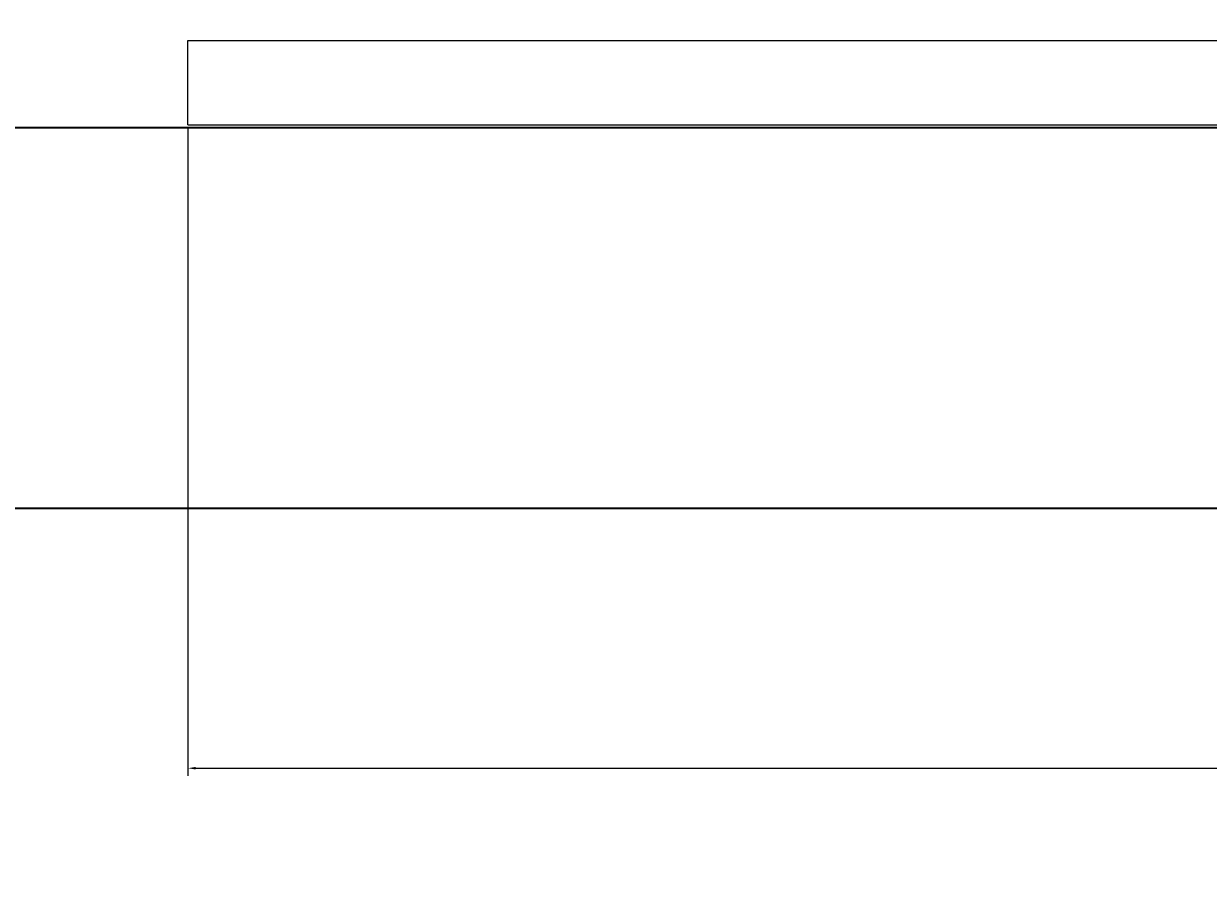
# Model space of a CAD drawing. Units: millimetres. Extents: x 27017497 to 27018854, y 7058029 to 7059154.
# Tile 19 of 91: x 27017651 to 27017679, y 7058124 to 7058144. Entities that reach past the tile are written whole.
import ezdxf

# ---------------------------------------------------------------- set-up
doc = ezdxf.new("R2010")
doc.units = ezdxf.units.MM
for name, color, linetype, lineweight in [('A-ANNO-DIMS', 2, 'Continuous', 18), ('A-FURN', 8, 'Continuous', 18), ('A-WALL', 7, 'Continuous', 35)]:
    doc.layers.add(name, color=color, linetype=linetype, lineweight=lineweight)
doc.styles.get("Standard").update_dxf_attribs({"font": 'arial.ttf'})
doc.dimstyles.get("Standard").update_dxf_attribs({"dimtxt": 0.18, "dimasz": 0.18, "dimexe": 0.18, "dimexo": 0.0625, "dimgap": 0.09, "dimtad": 0, "dimtih": 1, "dimtoh": 1, "dimdec": 4, "dimzin": 0, "dimdsep": 46, "dimtxsty": 'Standard', "dimcen": 0.09, "dimadec": 0, "dimazin": 0, "dimtfac": 1, "dimtdec": 4, "dimtofl": 0, "dimtmove": 0, "dimatfit": 3, "dimfxl": 1, "dimtolj": 1, "dimtzin": 0, "dimarcsym": 0})

# ---------------------------------------------------------------- blocks, each defined once
blk = doc.blocks.new('CAMMAT')
for p, q in [((1.27313, 0), (-1.27313, 0)), ((1.27313, 0), (1.27313, -0.05)), ((1.27313, -0.05), (-1.27313, -0.05))]:
    blk.add_line(p, q)
blk = doc.blocks.new('*D25')
at = {"layer": 'A-ANNO-DIMS', "color": 0, "lineweight": -2, "transparency": 16777216}
for p, q in [((27017654.932, 7058141.917), (27017654.932, 7058126.587)), ((27017756.349, 7058141.917), (27017756.349, 7058126.587)), ((27017655.112, 7058126.767), (27017704.753, 7058126.767)), ((27017756.169, 7058126.767), (27017706.528, 7058126.767))]:
    blk.add_line(p, q, dxfattribs=at)
at = {"layer": 'A-ANNO-DIMS', "color": 0, "transparency": 16777216}
for points in [[(27017655.112, 7058126.797), (27017655.112, 7058126.737), (27017654.932, 7058126.767)], [(27017756.169, 7058126.797), (27017756.169, 7058126.737), (27017756.349, 7058126.767)]]:
    blk.add_solid(points, dxfattribs=at)
at = {"layer": 'Defpoints', "color": 0, "transparency": 16777216}
for p in [(27017654.932, 7058141.98), (27017756.349, 7058141.98), (27017654.932, 7058126.767)]:
    blk.add_point(p, dxfattribs=at)
at = {"layer": 'A-ANNO-DIMS', "color": 0, "transparency": 16777216, "insert": (27017705.64, 7058126.767), "char_height": 0.18, "attachment_point": 5}
blk.add_mtext('\\A1;BED 101 TYP.', dxfattribs=at)
blk = doc.blocks.new('*D47')
at = {"layer": 'A-ANNO-DIMS', "color": 0, "lineweight": -2, "transparency": 16777216}
for p, q in [((27017561.166, 7058294.35), (27017561.166, 7058028.6)), ((27018790.606, 7058294.35), (27018790.606, 7058028.6)), ((27017561.346, 7058028.78), (27018175.431, 7058028.78)), ((27018790.426, 7058028.78), (27018176.341, 7058028.78))]:
    blk.add_line(p, q, dxfattribs=at)
at = {"layer": 'A-ANNO-DIMS', "color": 0, "transparency": 16777216}
for points in [[(27017561.346, 7058028.81), (27017561.346, 7058028.75), (27017561.166, 7058028.78)], [(27018790.426, 7058028.81), (27018790.426, 7058028.75), (27018790.606, 7058028.78)]]:
    blk.add_solid(points, dxfattribs=at)
at = {"layer": 'Defpoints', "color": 0, "transparency": 16777216}
for p in [(27017561.166, 7058294.412), (27018790.606, 7058294.412), (27018790.606, 7058028.78)]:
    blk.add_point(p, dxfattribs=at)
at = {"layer": 'A-ANNO-DIMS', "color": 0, "transparency": 16777216, "insert": (27018175.886, 7058028.78), "char_height": 0.18, "attachment_point": 5}
blk.add_mtext('\\A1;1229.4', dxfattribs=at)
blk = doc.blocks.new('*D48')
at = {"layer": 'A-ANNO-DIMS', "color": 0, "lineweight": -2, "transparency": 16777216}
for p, q in [((27018463.498, 7058622.912), (27017497.536, 7058622.912)), ((27017497.716, 7058622.732), (27017497.716, 7058357.753)), ((27017497.716, 7058092.41), (27017497.716, 7058357.389)), ((27018555.129, 7058092.23), (27017497.536, 7058092.23))]:
    blk.add_line(p, q, dxfattribs=at)
at = {"layer": 'A-ANNO-DIMS', "color": 0, "transparency": 16777216}
for points in [[(27017497.686, 7058622.732), (27017497.746, 7058622.732), (27017497.716, 7058622.912)], [(27017497.686, 7058092.41), (27017497.746, 7058092.41), (27017497.716, 7058092.23)]]:
    blk.add_solid(points, dxfattribs=at)
at = {"layer": 'Defpoints', "color": 0, "transparency": 16777216}
for p in [(27018463.561, 7058622.912), (27017497.716, 7058092.23), (27018555.192, 7058092.23)]:
    blk.add_point(p, dxfattribs=at)
at = {"layer": 'A-ANNO-DIMS', "color": 0, "transparency": 16777216, "insert": (27017497.716, 7058357.571), "char_height": 0.18, "attachment_point": 5}
blk.add_mtext('\\A1;530.7', dxfattribs=at)

msp = doc.modelspace()

# ---------------------------------------------------------------- linework, layer by layer
at = {"layer": 'A-WALL'}
for p, q in [((27017622.666, 7058141.912), (27017802.166, 7058141.912)), ((27017613.666, 7058132.912), (27017802.166, 7058132.912)), ((27017613.666, 7058132.912), (27017802.166, 7058132.912))]:
    msp.add_line(p, q, dxfattribs=at)

# ---------------------------------------------------------------- block references
at = {"layer": 'A-FURN', "xscale": 39.82996475819422, "yscale": 39.82996475819422, "zscale": 39.82996475819422, "rotation": 180}
msp.add_blockref('CAMMAT', (27017705.64, 7058141.98), dxfattribs=at)

# ---------------------------------------------------------------- dimensions: what is measured, and where the dimension line sits
at = {"layer": 'A-ANNO-DIMS'}
dim = msp.add_linear_dim(base=(27017497.716, 7058092.23), p1=(27018463.561, 7058622.912), p2=(27018555.192, 7058092.23), angle=90, dimstyle='Standard', override={"dimdec": 1, "dimlfac": 1, "dimrnd": 0, "dimzin": 0, "dimdsep": 46, "dimlunit": 2}, dxfattribs=at)
dim.commit()
dim.dimension.update_dxf_attribs({"geometry": '*D48', "text_midpoint": (27017497.716, 7058357.571)})
dim = msp.add_linear_dim(base=(27018790.606, 7058028.78), p1=(27017561.166, 7058294.412), p2=(27018790.606, 7058294.412), dimstyle='Standard', override={"dimdec": 1, "dimlfac": 1, "dimrnd": 0, "dimzin": 0, "dimdsep": 46, "dimlunit": 2}, dxfattribs=at)
dim.commit()
dim.dimension.update_dxf_attribs({"geometry": '*D47', "text_midpoint": (27018175.886, 7058028.78)})
dim = msp.add_linear_dim(base=(27017654.932, 7058126.767), p1=(27017756.349, 7058141.98), p2=(27017654.932, 7058141.98), angle=180, text='BED <> TYP.', dimstyle='Standard', override={"dimdec": 0, "dimlfac": 1, "dimrnd": 0, "dimzin": 0, "dimdsep": 46, "dimlunit": 2}, dxfattribs=at)
dim.commit()
dim.dimension.update_dxf_attribs({"geometry": '*D25', "text_midpoint": (27017705.64, 7058126.767)})

doc.saveas('drawing.dxf')
